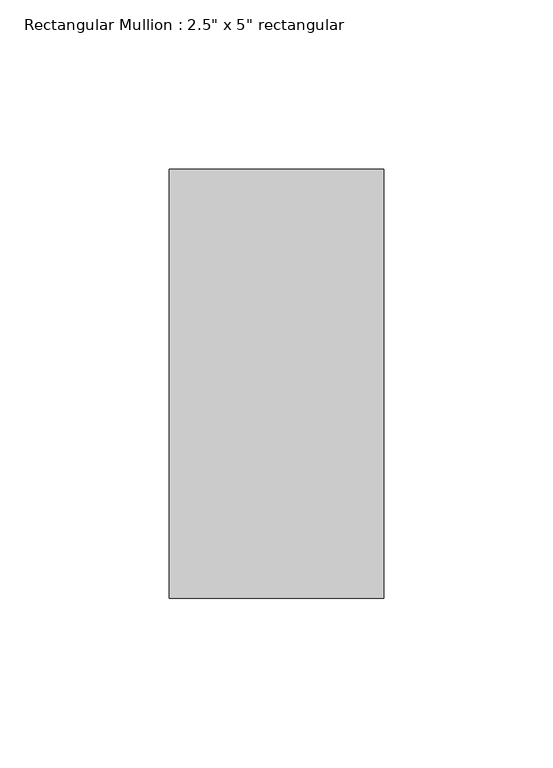
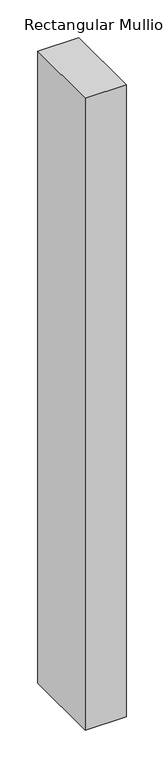
"""IFC4 building model written with IfcOpenShell, lengths in millimetres: member geometry."""

from ifc_helpers import new_model, si_unit, frame, origin, place, context, project, spatial, polyline, outline, extrude, source, transform, mapped, element, save


def member_9ad71e68(model_context):
    return source(origin(), model_context, "Body", "SweptSolid", [
        extrude(outline(polyline([(0.0, 63.5), (0.0, -63.5), (-63.5, -63.5), (-63.5, 63.5), (0.0, 63.5)])), frame((0.0, 0.0, -1028.434107), z_axis=(0.0, 0.0, 1.0), x_axis=(1.0, 0.0, 0.0)), (0.0, 0.0, 1.0), 1028.434107),
    ])


if __name__ == "__main__":
    model = new_model("IFC4")
    model_context = context("Model", 3, world=origin())
    ifc_project = project(units=[si_unit("LENGTHUNIT", "METRE", prefix="MILLI")], contexts=[model_context])
    site = spatial("IfcSite", under=ifc_project)
    building = spatial("IfcBuilding", under=site)
    placement = place(None, origin())
    member_shape = member_9ad71e68(model_context)
    element("IfcMember", 1, ObjectType="Rectangular Mullion : 2.5\" x 5\" rectangular", at=placement, inside=building, context=model_context, shape_type="MappedRepresentation", body=[
        mapped(member_shape, transform((0.0, 0.0, 0.0), x_axis=(1.0, 0.0, 0.0), y_axis=(0.0, 1.0, 0.0), z_axis=(0.0, 0.0, 1.0))),
    ])
    save(model, "model.ifc")

# Revit data of these elements
# Type "Rectangular Mullion : 2.5\" x 5\" rectangular"
#   built-in parameter 1007304 = 0.416667 (stored number, unit not read)
#   built-in parameter 1007301 = 0.104167 (stored number, unit not read)
#   built-in parameter 1007300 = 0.104167 (stored number, unit not read)
# Element 1 (IfcMember, "Rectangular Mullion : 2.5\" x 5\" rectangular")
#   Materials on its faces: "Roofing, EPDM Membrane"
# Materials
#   "Roofing, EPDM Membrane": class "Generic", colour RGB 127 127 127, transparency 0, Description = "EPDM roof membrane", Cost = 0
